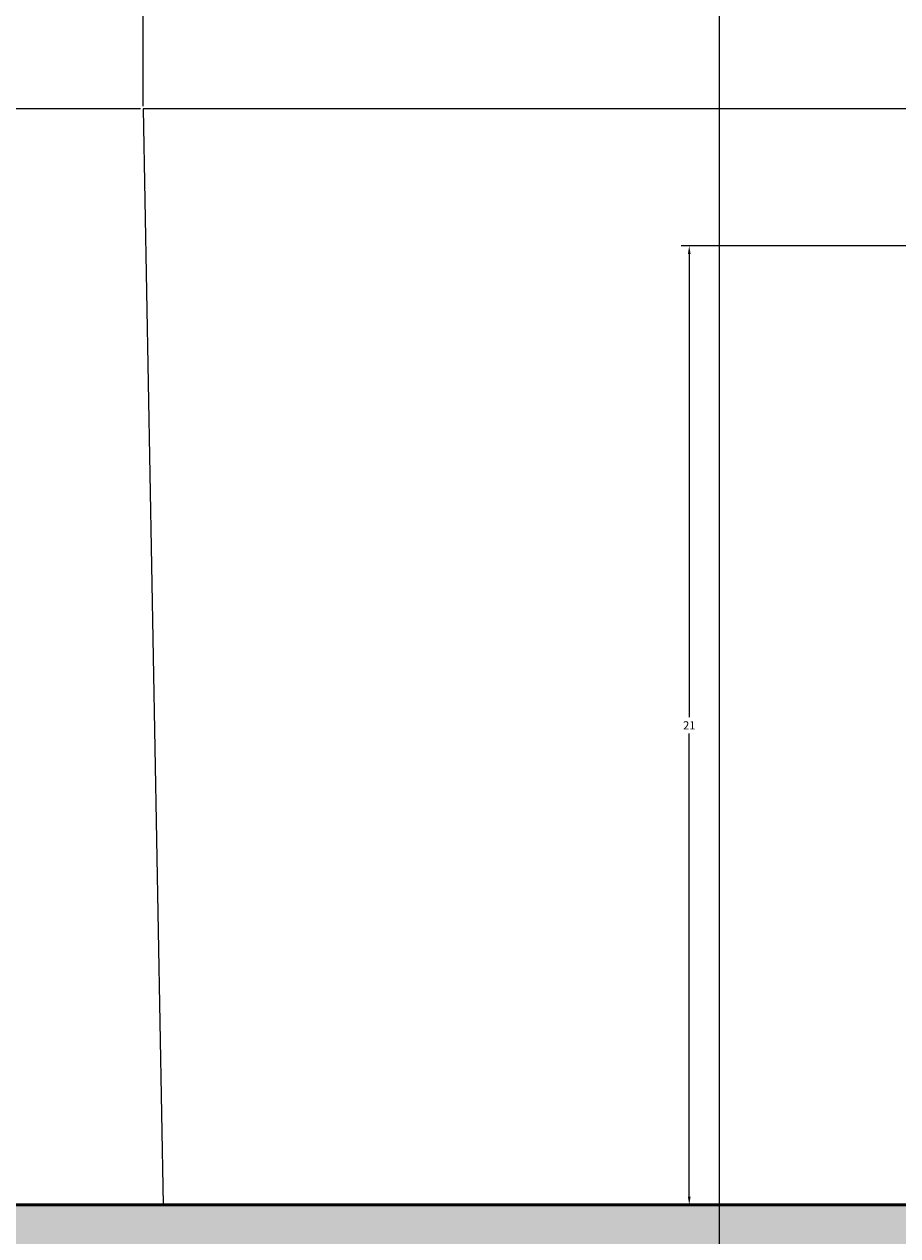
# Model space of a CAD drawing. Units: inches. Extents: x 2231 to 2461, y 2045 to 2455.
# Tile 16 of 95: x 2346 to 2365, y 2072 to 2099. Entities that reach past the tile are written whole.
import ezdxf

# ---------------------------------------------------------------- set-up
doc = ezdxf.new("R2010")
doc.units = ezdxf.units.IN
for name, color, linetype, lineweight in [('A-ANNO-DIMS', 2, 'Continuous', 18), ('A-FLOR-CASE', 8, 'Continuous', 25), ('A-WALL', 7, 'Continuous', 50)]:
    doc.layers.add(name, color=color, linetype=linetype, lineweight=lineweight)
doc.layers.add('A-WALL-PATT', color=18, linetype='Continuous', lineweight=13, true_color=0x000000)
doc.styles.get("Standard").update_dxf_attribs({"font": 'arial.ttf'})
doc.dimstyles.get("Standard").update_dxf_attribs({"dimtxt": 0.18, "dimasz": 0.18, "dimexe": 0.18, "dimexo": 0.0625, "dimgap": 0.09, "dimtad": 0, "dimtih": 1, "dimtoh": 1, "dimdec": 4, "dimzin": 0, "dimdsep": 46, "dimtxsty": 'Standard', "dimcen": 0.09, "dimadec": 0, "dimazin": 0, "dimtfac": 1, "dimtdec": 4, "dimtofl": 0, "dimtmove": 0, "dimatfit": 3, "dimfxl": 1, "dimtolj": 1, "dimtzin": 0, "dimarcsym": 0})

# ---------------------------------------------------------------- blocks, each defined once
blk = doc.blocks.new('*D30')
at = {"layer": 'A-ANNO-DIMS', "color": 0, "lineweight": -2, "transparency": 16777216}
for p, q in [((2365.477, 2093.833), (2359.96, 2093.833)), ((2360.14, 2093.653), (2360.14, 2083.513)), ((2360.14, 2073.013), (2360.14, 2083.152)), ((2365.477, 2072.833), (2359.96, 2072.833))]:
    blk.add_line(p, q, dxfattribs=at)
at = {"layer": 'A-ANNO-DIMS', "color": 0, "transparency": 16777216}
for points in [[(2360.11, 2093.653), (2360.17, 2093.653), (2360.14, 2093.833)], [(2360.11, 2073.013), (2360.17, 2073.013), (2360.14, 2072.833)]]:
    blk.add_solid(points, dxfattribs=at)
at = {"layer": 'Defpoints', "color": 0, "transparency": 16777216}
for p in [(2365.54, 2093.833), (2360.14, 2072.833), (2365.54, 2072.833)]:
    blk.add_point(p, dxfattribs=at)
at = {"layer": 'A-ANNO-DIMS', "color": 0, "transparency": 16777216, "insert": (2360.14, 2083.333), "char_height": 0.18, "attachment_point": 5}
blk.add_mtext('\\A1;21', dxfattribs=at)
blk = doc.blocks.new('*D52')
at = {"layer": 'A-ANNO-DIMS', "color": 0, "lineweight": -2, "transparency": 16777216}
for p, q in [((2330.794, 2306.77), (2330.794, 2044.803)), ((2360.794, 2306.77), (2360.794, 2044.803)), ((2330.974, 2044.983), (2345.575, 2044.983)), ((2360.614, 2044.983), (2346.012, 2044.983))]:
    blk.add_line(p, q, dxfattribs=at)
at = {"layer": 'A-ANNO-DIMS', "color": 0, "transparency": 16777216}
for points in [[(2330.974, 2045.013), (2330.974, 2044.953), (2330.794, 2044.983)], [(2360.614, 2045.013), (2360.614, 2044.953), (2360.794, 2044.983)]]:
    blk.add_solid(points, dxfattribs=at)
at = {"layer": 'Defpoints', "color": 0, "transparency": 16777216}
for p in [(2330.794, 2306.833), (2360.794, 2306.833), (2360.794, 2044.983)]:
    blk.add_point(p, dxfattribs=at)
at = {"layer": 'A-ANNO-DIMS', "color": 0, "transparency": 16777216, "insert": (2345.794, 2044.983), "char_height": 0.18, "attachment_point": 5}
blk.add_mtext('\\A1;30', dxfattribs=at)
blk = doc.blocks.new('*D66')
at = {"layer": 'A-ANNO-DIMS', "color": 0, "lineweight": -2, "transparency": 16777216}
for p, q in [((2348.189, 2096.895), (2348.189, 2454.645)), ((2408.794, 2096.895), (2408.794, 2454.645)), ((2348.369, 2454.465), (2378.167, 2454.465)), ((2408.614, 2454.465), (2378.815, 2454.465))]:
    blk.add_line(p, q, dxfattribs=at)
at = {"layer": 'A-ANNO-DIMS', "color": 0, "transparency": 16777216}
for points in [[(2348.369, 2454.495), (2348.369, 2454.435), (2348.189, 2454.465)], [(2408.614, 2454.495), (2408.614, 2454.435), (2408.794, 2454.465)]]:
    blk.add_solid(points, dxfattribs=at)
at = {"layer": 'Defpoints', "color": 0, "transparency": 16777216}
for p in [(2408.794, 2454.465), (2348.189, 2096.833), (2408.794, 2096.833)]:
    blk.add_point(p, dxfattribs=at)
at = {"layer": 'A-ANNO-DIMS', "color": 0, "transparency": 16777216, "insert": (2378.491, 2454.465), "char_height": 0.18, "attachment_point": 5}
blk.add_mtext('\\A1;60.6', dxfattribs=at)
blk = doc.blocks.new('*D67')
at = {"layer": 'A-ANNO-DIMS', "color": 0, "lineweight": -2, "transparency": 16777216}
for p, q in [((2348.126, 2096.833), (2230.981, 2096.833)), ((2231.161, 2096.653), (2231.161, 2085.013)), ((2231.161, 2073.013), (2231.161, 2084.652)), ((2348.559, 2072.833), (2230.981, 2072.833))]:
    blk.add_line(p, q, dxfattribs=at)
at = {"layer": 'A-ANNO-DIMS', "color": 0, "transparency": 16777216}
for points in [[(2231.131, 2096.653), (2231.191, 2096.653), (2231.161, 2096.833)], [(2231.131, 2073.013), (2231.191, 2073.013), (2231.161, 2072.833)]]:
    blk.add_solid(points, dxfattribs=at)
at = {"layer": 'Defpoints', "color": 0, "transparency": 16777216}
for p in [(2348.189, 2096.833), (2231.161, 2072.833), (2348.622, 2072.833)]:
    blk.add_point(p, dxfattribs=at)
at = {"layer": 'A-ANNO-DIMS', "color": 0, "transparency": 16777216, "insert": (2231.161, 2084.833), "char_height": 0.18, "attachment_point": 5}
blk.add_mtext('\\A1;24', dxfattribs=at)
blk = doc.blocks.new('*D69')
at = {"layer": 'A-ANNO-DIMS', "color": 0, "lineweight": -2, "transparency": 16777216}
for p, q in [((2340.667, 2189.285), (2340.667, 2044.803)), ((2394.794, 2186.77), (2394.794, 2044.803)), ((2340.847, 2044.983), (2367.337, 2044.983)), ((2394.614, 2044.983), (2368.124, 2044.983))]:
    blk.add_line(p, q, dxfattribs=at)
at = {"layer": 'A-ANNO-DIMS', "color": 0, "transparency": 16777216}
for points in [[(2340.847, 2045.013), (2340.847, 2044.953), (2340.667, 2044.983)], [(2394.614, 2045.013), (2394.614, 2044.953), (2394.794, 2044.983)]]:
    blk.add_solid(points, dxfattribs=at)
at = {"layer": 'Defpoints', "color": 0, "transparency": 16777216}
for p in [(2340.667, 2189.348), (2394.794, 2186.833), (2394.794, 2044.983)]:
    blk.add_point(p, dxfattribs=at)
at = {"layer": 'A-ANNO-DIMS', "color": 0, "transparency": 16777216, "insert": (2367.73, 2044.983), "char_height": 0.18, "attachment_point": 5}
blk.add_mtext('\\A1;54.13', dxfattribs=at)

msp = doc.modelspace()

# ---------------------------------------------------------------- hatches: boundary and pattern name
at = {"layer": 'A-WALL-PATT'}
h = msp.add_hatch(color=256, dxfattribs=at)
h.dxf.hatch_style = 1
h.paths.add_polyline_path([(2441.7935, 2269.1535), (2432.7935, 2269.1535), (2432.7935, 2186.8328), (2396.7935, 2186.8328), (2396.7935, 2286.8328), (2394.7935, 2286.8328), (2394.7935, 2186.8328), (2334.7935, 2186.8328), (2334.7935, 2182.8328), (2432.7935, 2182.8328), (2432.7935, 2072.8328), (2416.6639, 2072.8328), (2416.6639, 2063.8328), (2441.7935, 2063.8328)])
h.paths.add_polyline_path([(2368.6639, 2072.8328), (2367.04, 2072.8328), (2330.7942, 2072.8328), (2330.7397, 2063.8328), (2368.6639, 2063.8328)])
h.paths.add_polyline_path([(2300.7392, 2068.3328), (2300.7392, 2072.8328), (2298.7935, 2072.8328), (2294.7935, 2072.8328), (2258.7935, 2072.8328), (2258.7935, 2120.8328), (2294.7935, 2120.8328), (2298.7935, 2120.8328), (2298.7935, 2128.8328), (2294.7935, 2128.8328), (2294.7935, 2124.8328), (2258.7935, 2124.8328), (2258.7935, 2182.8328), (2294.7935, 2182.8328), (2294.7935, 2174.8328), (2298.7935, 2174.8328), (2298.7935, 2182.8328), (2304.7935, 2182.8328), (2304.7935, 2186.8328), (2258.7935, 2186.8328), (2258.7935, 2221.999), (2249.7935, 2221.999), (2249.7935, 2063.8328), (2300.7392, 2063.8328)])
h.paths.add_polyline_path([(2391.9338, 2435.8328), (2333.82, 2435.8328), (2333.82, 2426.8328), (2368.7935, 2426.8328), (2368.7935, 2374.9508), (2368.7935, 2370.8328), (2372.3935, 2370.8328), (2372.7935, 2370.8328), (2372.7935, 2426.8328), (2391.9338, 2426.8328)])
h.paths.add_polyline_path([(2441.7935, 2435.8328), (2415.9338, 2435.8328), (2415.9338, 2426.8328), (2432.7935, 2426.8328), (2432.7935, 2334.8328), (2372.7935, 2334.8328), (2372.7935, 2346.8328), (2368.7935, 2346.8328), (2368.7935, 2306.8328), (2360.7935, 2306.8328), (2360.7935, 2302.8328), (2368.7935, 2302.8328), (2372.7935, 2302.8328), (2372.7935, 2330.8328), (2432.7935, 2330.8328), (2432.7935, 2317.1535), (2441.7935, 2317.1535)])
h.paths.add_polyline_path([(2285.82, 2435.8328), (2249.7935, 2435.8328), (2249.7935, 2269.999), (2258.7935, 2269.999), (2258.7935, 2302.8328), (2318.8168, 2302.8328), (2330.7935, 2302.8328), (2330.7935, 2306.8328), (2258.7935, 2306.8328), (2258.7935, 2426.8328), (2285.82, 2426.8328)])

# ---------------------------------------------------------------- linework, layer by layer
at = {"layer": 'A-FLOR-CASE'}
for p, q in [((2408.7935, 2096.8328), (2348.1888, 2096.8328)), ((2348.1888, 2096.8328), (2348.6219, 2072.8328))]:
    msp.add_line(p, q, dxfattribs=at)
at = {"layer": 'A-WALL'}
msp.add_line((2432.7935, 2072.8328), (2330.7942, 2072.8328), dxfattribs=at)

# ---------------------------------------------------------------- dimensions: what is measured, and where the dimension line sits
at = {"layer": 'A-ANNO-DIMS'}
for base, p1, p2, override, picture, middle in [((2408.7935, 2454.4653), (2348.1888, 2096.8328), (2408.7935, 2096.8328), {"dimdec": 1, "dimlfac": 1, "dimrnd": 0, "dimzin": 0, "dimdsep": 46, "dimlunit": 2}, '*D66', (2378.4912, 2454.4653)), ((2360.7935, 2044.9825), (2330.7935, 2306.8328), (2360.7935, 2306.8328), {"dimdec": 0, "dimlfac": 1, "dimrnd": 0, "dimzin": 0, "dimdsep": 46, "dimlunit": 2}, '*D52', (2345.7935, 2044.9825)), ((2394.7935, 2044.9825), (2340.6673, 2189.3477), (2394.7935, 2186.8328), {"dimdec": 2, "dimlfac": 1, "dimrnd": 0, "dimzin": 0, "dimdsep": 46, "dimlunit": 2}, '*D69', (2367.7304, 2044.9825))]:
    dim = msp.add_linear_dim(base=base, p1=p1, p2=p2, dimstyle='Standard', override=override, dxfattribs=at)
    dim.commit()
    dim.dimension.update_dxf_attribs({"geometry": picture, "text_midpoint": middle})
for base, p1, p2, angle, picture, middle in [((2231.161, 2072.8328), (2348.1888, 2096.8328), (2348.6219, 2072.8328), 90, '*D67', (2231.161, 2084.8328)), ((2360.14, 2072.8328), (2365.54, 2093.8328), (2365.54, 2072.8328), 270, '*D30', (2360.14, 2083.3328))]:
    dim = msp.add_linear_dim(base=base, p1=p1, p2=p2, angle=angle, dimstyle='Standard', override={"dimdec": 0, "dimlfac": 1, "dimrnd": 0, "dimzin": 0, "dimdsep": 46, "dimlunit": 2}, dxfattribs=at)
    dim.commit()
    dim.dimension.update_dxf_attribs({"geometry": picture, "text_midpoint": middle})

doc.saveas('drawing.dxf')
